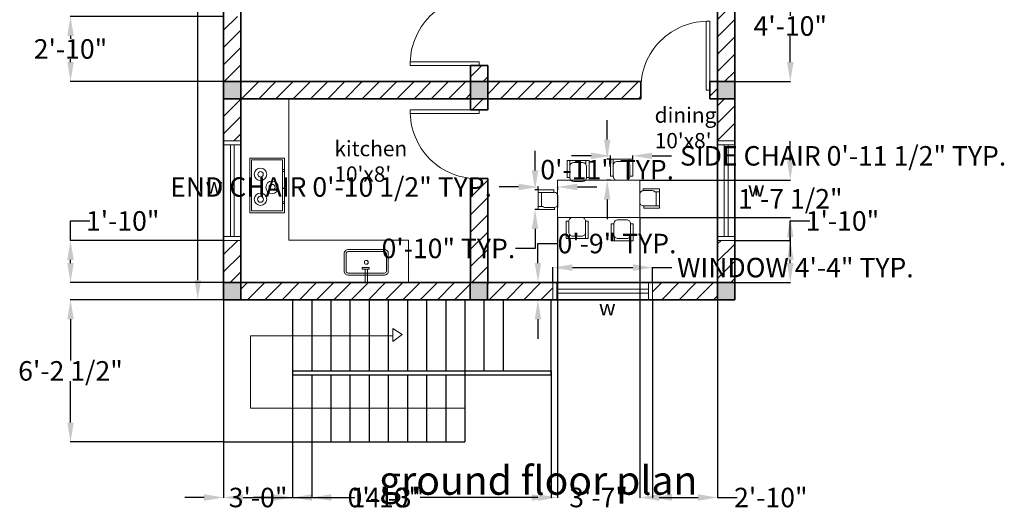
# Model space of a CAD drawing. Units: inches. Extents: x 1222 to 2611, y 176 to 793.
# Tile 1 of 5: x 1222 to 1737, y 176 to 433. Entities that reach past the tile are written whole.
import ezdxf

# ---------------------------------------------------------------- set-up
doc = ezdxf.new("R2010")
doc.units = ezdxf.units.IN
doc.header["$MEASUREMENT"] = 0
for name, color, linetype, lineweight in [('A-ANNO-DIMS', 2, 'Continuous', 18), ('A-ANNO-SYMB', 7, 'Continuous', 18), ('A-ANNO-TEXT', 7, 'Continuous', 25), ('A-AREA-IDEN', 7, 'Continuous', 25), ('A-COLS', 7, 'Continuous', 35), ('A-COLS-PATT', 18, 'Continuous', 13), ('A-DOOR', 3, 'Continuous', 18), ('A-EQPM', 8, 'Continuous', 18), ('A-FLOR-CASE', 9, 'Continuous', 18), ('A-FLOR-FIXT', 9, 'Continuous', 18), ('A-FLOR-STRS', 7, 'Continuous', 25), ('A-FURN', 8, 'Continuous', 18), ('A-GLAZ', 4, 'Continuous', 18), ('A-WALL', 7, 'Continuous', 35), ('A-WALL-PATT', 30, 'Continuous', 13)]:
    doc.layers.add(name, color=color, linetype=linetype, lineweight=lineweight)
doc.styles.get("Standard").update_dxf_attribs({"font": 'arial.ttf'})
doc.dimstyles.get("Standard").update_dxf_attribs({"dimtxt": 10.18, "dimasz": 10.18, "dimexe": 0.18, "dimexo": 0.0625, "dimgap": 0.09, "dimtad": 0, "dimtih": 1, "dimtoh": 1, "dimdec": 0, "dimzin": 0, "dimdsep": 46, "dimlunit": 3, "dimtxsty": 'Standard', "dimcen": 0.09, "dimadec": 0, "dimazin": 0, "dimtfac": 1, "dimtdec": 0, "dimtofl": 0, "dimtmove": 0, "dimatfit": 3, "dimfxl": 1, "dimtolj": 1, "dimtzin": 0, "dimarcsym": 0})

# ---------------------------------------------------------------- blocks, each defined once
blk = doc.blocks.new('*D10')
at = {"layer": 'A-ANNO-DIMS', "color": 0, "lineweight": -2, "transparency": 16777216}
for p, q in [((1328.74, 730.54), (1315.1, 730.54)), ((1315.28, 720.36), (1315.28, 513.8)), ((1315.28, 296.65), (1315.28, 503.21)), ((1328.74, 286.47), (1315.1, 286.47))]:
    blk.add_line(p, q, dxfattribs=at)
at = {"layer": 'A-ANNO-DIMS', "color": 0, "transparency": 16777216}
for points in [[(1313.58, 720.36), (1316.97, 720.36), (1315.28, 730.54)], [(1313.58, 296.65), (1316.97, 296.65), (1315.28, 286.47)]]:
    blk.add_solid(points, dxfattribs=at)
at = {"layer": 'Defpoints', "color": 0, "transparency": 16777216}
for p in [(1315.28, 730.54), (1328.8, 730.54), (1328.8, 286.47)]:
    blk.add_point(p, dxfattribs=at)
at = {"layer": 'A-ANNO-DIMS', "color": 0, "transparency": 16777216, "insert": (1315.28, 508.5), "char_height": 10.18, "attachment_point": 5}
blk.add_mtext("\\A1;37'", dxfattribs=at)
blk = doc.blocks.new('DOOR-SWING-36IN')
for p, q in [((34.01, 0), (34.01, 36)), ((36.01, 0), (36.01, 36)), ((34.01, 0), (36.01, 0))]:
    blk.add_line(p, q)
blk.add_arc((35.01, 1), 35.01, 88.3634, 181.6366)
blk = doc.blocks.new('WINDOW-48IN-PLAN')
for p, q in [((0, 0), (0, 9)), ((2, 0), (2, 9)), ((2, 5.5), (50, 5.5)), ((50, 0), (50, 9)), ((52, 0), (52, 9)), ((2, 3.5), (50, 3.5))]:
    blk.add_line(p, q)
blk = doc.blocks.new('COLUMN-9X9IN')
blk.add_lwpolyline([(0, 9), (9, 9), (9, 0), (0, 0)], close=True)
blk = doc.blocks.new('CHAIR-DINING-SIDE')
for points in [[(2.02, 10.94), (2.02, 10.94), (0, 10.94), (0, 10.94), (0, 4.9), (0, 4.9)], [(9.79, 9.21), (9.79, 9.21), (9.79, 10.94), (9.79, 10.94), (2.02, 10.94), (2.02, 10.94)], [(9.79, 8.89), (9.79, 10.94), (9.79, 10.94), (11.58, 10.94), (11.58, 10.94), (11.58, 2.01), (11.58, 2.01), (10.11, 2.01)]]:
    blk.add_lwpolyline(points)
blk.add_lwpolyline([(0, 10.94), (0, 10.94), (1.43, 10.94), (1.43, 10.94), (1.43, 2), (1.43, 2), (0, 2), (0, 2)], close=True)
blk.add_lwpolyline([(10.11, 2, -0.414214), (8.11, 0), (3.43, 0, -0.414214), (1.43, 2), (1.43, 7.79, -0.414214), (3.43, 9.79), (8.11, 9.79, -0.414214), (10.11, 7.79)], format="xyb", close=True)
blk = doc.blocks.new('CHAIR-DINING-END')
blk.add_lwpolyline([(2.18, 1.24), (2, 1.24, -0.414214), (0, 3.24), (0, 7.18, -0.414214), (2, 9.18), (6.51, 9.18, -0.198912), (7.92, 8.59)], format="xyb")
blk.add_lwpolyline([(1.78, 9.17), (1.78, 10.19), (1.78, 10.19), (10.36, 10.19), (10.36, 10.19), (10.36, 8.59), (10.36, 8.59), (7.92, 8.59)])
for points in [[(8.51, 8.59), (8.51, 8.59), (10.36, 8.59), (10.36, 8.59), (10.36, 1.33), (10.36, 1.33), (8.51, 1.33), (8.51, 1.33)], [(10.36, 1.33), (10.36, 1.33), (2.18, 1.33), (2.18, 1.33), (2.18, 0), (2.18, 0), (10.36, 0), (10.36, 0)]]:
    blk.add_lwpolyline(points, close=True)
blk = doc.blocks.new('*D18')
at = {"layer": 'A-ANNO-DIMS', "color": 0, "lineweight": -2, "transparency": 16777216}
for p, q in [((1500.8, 295.54), (1500.8, 303.45)), ((1510.98, 303.27), (1542.62, 303.27)), ((1552.8, 295.54), (1552.8, 303.45)), ((1552.8, 303.27), (1562.98, 303.27))]:
    blk.add_line(p, q, dxfattribs=at)
at = {"layer": 'A-ANNO-DIMS', "color": 0, "transparency": 16777216}
for points in [[(1510.98, 304.97), (1510.98, 301.58), (1500.8, 303.27)], [(1542.62, 304.97), (1542.62, 301.58), (1552.8, 303.27)]]:
    blk.add_solid(points, dxfattribs=at)
at = {"layer": 'Defpoints', "color": 0, "transparency": 16777216}
for p in [(1552.8, 303.27), (1500.8, 295.47), (1552.8, 295.47)]:
    blk.add_point(p, dxfattribs=at)
at = {"layer": 'A-ANNO-DIMS', "color": 0, "transparency": 16777216, "insert": (1627.48, 303.27), "char_height": 10.18, "attachment_point": 5}
blk.add_mtext('\\A1;WINDOW 4\'-4" TYP.', dxfattribs=at)
blk = doc.blocks.new('*D19')
at = {"layer": 'A-ANNO-DIMS', "color": 0, "lineweight": -2, "transparency": 16777216}
for p, q in [((1493, 305.65), (1493, 315.83)), ((1493, 315.83), (1503.18, 315.83)), ((1500.74, 295.47), (1492.82, 295.47)), ((1500.74, 286.47), (1492.82, 286.47)), ((1493, 276.29), (1493, 266.11))]:
    blk.add_line(p, q, dxfattribs=at)
at = {"layer": 'A-ANNO-DIMS', "color": 0, "transparency": 16777216}
for points in [[(1491.31, 305.65), (1494.7, 305.65), (1493, 295.47)], [(1491.31, 276.29), (1494.7, 276.29), (1493, 286.47)]]:
    blk.add_solid(points, dxfattribs=at)
at = {"layer": 'Defpoints', "color": 0, "transparency": 16777216}
for p in [(1493, 295.47), (1500.8, 295.47), (1500.8, 286.47)]:
    blk.add_point(p, dxfattribs=at)
at = {"layer": 'A-ANNO-DIMS', "color": 0, "transparency": 16777216, "insert": (1534.3, 315.83), "char_height": 10.18, "attachment_point": 5}
blk.add_mtext('\\A1;0\'-9" TYP.', dxfattribs=at)
blk = doc.blocks.new('*D22')
at = {"layer": 'A-ANNO-DIMS', "color": 0, "lineweight": -2, "transparency": 16777216}
for p, q in [((1520.73, 361.64), (1510.55, 361.64)), ((1530.91, 359.97), (1530.91, 361.82)), ((1542.48, 359.97), (1542.48, 361.82)), ((1552.66, 361.64), (1562.84, 361.64))]:
    blk.add_line(p, q, dxfattribs=at)
at = {"layer": 'A-ANNO-DIMS', "color": 0, "transparency": 16777216}
for points in [[(1520.73, 363.34), (1520.73, 359.95), (1530.91, 361.64)], [(1552.66, 363.34), (1552.66, 359.95), (1542.48, 361.64)]]:
    blk.add_solid(points, dxfattribs=at)
at = {"layer": 'Defpoints', "color": 0, "transparency": 16777216}
for p in [(1542.48, 361.64), (1530.91, 359.91), (1542.48, 359.91)]:
    blk.add_point(p, dxfattribs=at)
at = {"layer": 'A-ANNO-DIMS', "color": 0, "transparency": 16777216, "insert": (1652.42, 361.64), "char_height": 10.18, "attachment_point": 5}
blk.add_mtext('\\A1;SIDE CHAIR 0\'-11 1/2" TYP.', dxfattribs=at)
blk = doc.blocks.new('*D23')
at = {"layer": 'A-ANNO-DIMS', "color": 0, "lineweight": -2, "transparency": 16777216}
for p, q in [((1529.17, 370.09), (1529.17, 380.27)), ((1530.84, 359.91), (1528.99, 359.91)), ((1530.84, 348.96), (1528.99, 348.96)), ((1529.17, 338.78), (1529.17, 328.6))]:
    blk.add_line(p, q, dxfattribs=at)
at = {"layer": 'A-ANNO-DIMS', "color": 0, "transparency": 16777216}
for points in [[(1527.47, 370.09), (1530.87, 370.09), (1529.17, 359.91)], [(1527.47, 338.78), (1530.87, 338.78), (1529.17, 348.96)]]:
    blk.add_solid(points, dxfattribs=at)
at = {"layer": 'Defpoints', "color": 0, "transparency": 16777216}
for p in [(1529.17, 359.91), (1530.91, 359.91), (1530.91, 348.96)]:
    blk.add_point(p, dxfattribs=at)
at = {"layer": 'A-ANNO-DIMS', "color": 0, "transparency": 16777216, "insert": (1529.17, 354.43), "char_height": 10.18, "attachment_point": 5}
blk.add_mtext('\\A1;0\'-11" TYP.', dxfattribs=at)
blk = doc.blocks.new('*D24')
at = {"layer": 'A-ANNO-DIMS', "color": 0, "lineweight": -2, "transparency": 16777216}
for p, q in [((1482.85, 345.38), (1472.67, 345.38)), ((1493.03, 343.89), (1493.03, 345.56)), ((1503.39, 343.89), (1503.39, 345.56)), ((1513.57, 345.38), (1523.75, 345.38))]:
    blk.add_line(p, q, dxfattribs=at)
at = {"layer": 'A-ANNO-DIMS', "color": 0, "transparency": 16777216}
for points in [[(1482.85, 347.08), (1482.85, 343.68), (1493.03, 345.38)], [(1513.57, 347.08), (1513.57, 343.68), (1503.39, 345.38)]]:
    blk.add_solid(points, dxfattribs=at)
at = {"layer": 'Defpoints', "color": 0, "transparency": 16777216}
for p in [(1493.03, 345.38), (1493.03, 343.83), (1503.39, 343.83)]:
    blk.add_point(p, dxfattribs=at)
at = {"layer": 'A-ANNO-DIMS', "color": 0, "transparency": 16777216, "insert": (1384.92, 345.38), "char_height": 10.18, "attachment_point": 5}
blk.add_mtext('\\A1;END CHAIR 0\'-10 1/2" TYP.', dxfattribs=at)
blk = doc.blocks.new('*D25')
at = {"layer": 'A-ANNO-DIMS', "color": 0, "lineweight": -2, "transparency": 16777216}
for p, q in [((1491.48, 354.01), (1491.48, 364.19)), ((1492.97, 343.83), (1491.3, 343.83)), ((1492.97, 333.64), (1491.3, 333.64)), ((1491.48, 323.46), (1491.48, 313.28)), ((1491.48, 313.28), (1481.3, 313.28))]:
    blk.add_line(p, q, dxfattribs=at)
at = {"layer": 'A-ANNO-DIMS', "color": 0, "transparency": 16777216}
for points in [[(1489.78, 354.01), (1493.17, 354.01), (1491.48, 343.83)], [(1489.78, 323.46), (1493.17, 323.46), (1491.48, 333.64)]]:
    blk.add_solid(points, dxfattribs=at)
at = {"layer": 'Defpoints', "color": 0, "transparency": 16777216}
for p in [(1493.03, 343.83), (1491.48, 333.64), (1493.03, 333.64)]:
    blk.add_point(p, dxfattribs=at)
at = {"layer": 'A-ANNO-DIMS', "color": 0, "transparency": 16777216, "insert": (1446.22, 313.28), "char_height": 10.18, "attachment_point": 5}
blk.add_mtext('\\A1;0\'-10" TYP.', dxfattribs=at)
blk = doc.blocks.new('*D26')
at = {"layer": 'A-ANNO-DIMS', "color": 0, "lineweight": -2, "transparency": 16777216}
for p, q in [((1328.74, 286.47), (1248.62, 286.47)), ((1248.8, 276.29), (1248.8, 254.68)), ((1248.8, 222.35), (1248.8, 243.97)), ((1328.74, 212.17), (1248.62, 212.17))]:
    blk.add_line(p, q, dxfattribs=at)
at = {"layer": 'A-ANNO-DIMS', "color": 0, "transparency": 16777216}
for points in [[(1247.11, 276.29), (1250.5, 276.29), (1248.8, 286.47)], [(1247.11, 222.35), (1250.5, 222.35), (1248.8, 212.17)]]:
    blk.add_solid(points, dxfattribs=at)
at = {"layer": 'Defpoints', "color": 0, "transparency": 16777216}
for p in [(1328.8, 286.47), (1248.8, 212.17), (1328.8, 212.17)]:
    blk.add_point(p, dxfattribs=at)
at = {"layer": 'A-ANNO-DIMS', "color": 0, "transparency": 16777216, "insert": (1248.8, 249.32), "char_height": 10.18, "attachment_point": 5}
blk.add_mtext('\\A1;6\'-2 1/2"', dxfattribs=at)
blk = doc.blocks.new('*D27')
at = {"layer": 'A-ANNO-DIMS', "color": 0, "lineweight": -2, "transparency": 16777216}
for p, q in [((1328.8, 286.41), (1328.8, 182.99)), ((1499.95, 249.26), (1499.95, 182.99)), ((1338.98, 183.17), (1397.28, 183.17)), ((1489.77, 183.17), (1431.47, 183.17))]:
    blk.add_line(p, q, dxfattribs=at)
at = {"layer": 'A-ANNO-DIMS', "color": 0, "transparency": 16777216}
for points in [[(1338.98, 184.87), (1338.98, 181.47), (1328.8, 183.17)], [(1489.77, 184.87), (1489.77, 181.47), (1499.95, 183.17)]]:
    blk.add_solid(points, dxfattribs=at)
at = {"layer": 'Defpoints', "color": 0, "transparency": 16777216}
for p in [(1328.8, 286.47), (1499.95, 249.32), (1499.95, 183.17)]:
    blk.add_point(p, dxfattribs=at)
at = {"layer": 'A-ANNO-DIMS', "color": 0, "transparency": 16777216, "insert": (1414.38, 183.17), "char_height": 10.18, "attachment_point": 5}
blk.add_mtext('\\A1;14\'-3"', dxfattribs=at)
blk = doc.blocks.new('*D28')
at = {"layer": 'A-ANNO-DIMS', "color": 0, "lineweight": -2, "transparency": 16777216}
for p, q in [((1364.8, 212.11), (1364.8, 182.99)), ((1374.8, 212.11), (1374.8, 182.99)), ((1354.62, 183.17), (1344.44, 183.17)), ((1384.98, 183.17), (1395.16, 183.17))]:
    blk.add_line(p, q, dxfattribs=at)
at = {"layer": 'A-ANNO-DIMS', "color": 0, "transparency": 16777216}
for points in [[(1354.62, 184.87), (1354.62, 181.47), (1364.8, 183.17)], [(1384.98, 184.87), (1384.98, 181.47), (1374.8, 183.17)]]:
    blk.add_solid(points, dxfattribs=at)
at = {"layer": 'Defpoints', "color": 0, "transparency": 16777216}
for p in [(1364.8, 212.17), (1374.8, 212.17), (1374.8, 183.17)]:
    blk.add_point(p, dxfattribs=at)
at = {"layer": 'A-ANNO-DIMS', "color": 0, "transparency": 16777216, "insert": (1412.74, 183.17), "char_height": 10.18, "attachment_point": 5}
blk.add_mtext('\\A1;0\'-10"', dxfattribs=at)
blk = doc.blocks.new('*D29')
at = {"layer": 'A-ANNO-DIMS', "color": 0, "lineweight": -2, "transparency": 16777216}
for p, q in [((1328.8, 212.11), (1328.8, 182.99)), ((1364.8, 212.11), (1364.8, 182.99)), ((1318.62, 183.17), (1308.44, 183.17)), ((1374.98, 183.17), (1385.16, 183.17))]:
    blk.add_line(p, q, dxfattribs=at)
at = {"layer": 'A-ANNO-DIMS', "color": 0, "transparency": 16777216}
for points in [[(1318.62, 184.87), (1318.62, 181.47), (1328.8, 183.17)], [(1374.98, 184.87), (1374.98, 181.47), (1364.8, 183.17)]]:
    blk.add_solid(points, dxfattribs=at)
at = {"layer": 'Defpoints', "color": 0, "transparency": 16777216}
for p in [(1328.8, 212.17), (1364.8, 212.17), (1328.8, 183.17)]:
    blk.add_point(p, dxfattribs=at)
at = {"layer": 'A-ANNO-DIMS', "color": 0, "transparency": 16777216, "insert": (1346.8, 183.17), "char_height": 10.18, "attachment_point": 5}
blk.add_mtext('\\A1;3\'-0"', dxfattribs=at)
blk = doc.blocks.new('*D34')
at = {"layer": 'A-ANNO-DIMS', "color": 0, "lineweight": -2, "transparency": 16777216}
for p, q in [((1328.74, 434.47), (1248.62, 434.47)), ((1248.8, 424.29), (1248.8, 422.76)), ((1248.8, 410.65), (1248.8, 412.19)), ((1328.74, 400.47), (1248.62, 400.47))]:
    blk.add_line(p, q, dxfattribs=at)
at = {"layer": 'A-ANNO-DIMS', "color": 0, "transparency": 16777216}
for points in [[(1247.11, 424.29), (1250.5, 424.29), (1248.8, 434.47)], [(1247.11, 410.65), (1250.5, 410.65), (1248.8, 400.47)]]:
    blk.add_solid(points, dxfattribs=at)
at = {"layer": 'Defpoints', "color": 0, "transparency": 16777216}
for p in [(1248.8, 434.47), (1328.8, 434.47), (1328.8, 400.47)]:
    blk.add_point(p, dxfattribs=at)
at = {"layer": 'A-ANNO-DIMS', "color": 0, "transparency": 16777216, "insert": (1248.8, 417.47), "char_height": 10.18, "attachment_point": 5}
blk.add_mtext('\\A1;2\'-10"', dxfattribs=at)
blk = doc.blocks.new('*D35')
at = {"layer": 'A-ANNO-DIMS', "color": 0, "lineweight": -2, "transparency": 16777216}
for p, q in [((1248.8, 317.47), (1248.8, 327.65)), ((1248.8, 327.65), (1258.98, 327.65)), ((1328.74, 317.47), (1248.62, 317.47)), ((1248.8, 305.65), (1248.8, 307.29)), ((1337.74, 295.47), (1248.62, 295.47))]:
    blk.add_line(p, q, dxfattribs=at)
at = {"layer": 'A-ANNO-DIMS', "color": 0, "transparency": 16777216}
for points in [[(1247.11, 307.29), (1250.5, 307.29), (1248.8, 317.47)], [(1247.11, 305.65), (1250.5, 305.65), (1248.8, 295.47)]]:
    blk.add_solid(points, dxfattribs=at)
at = {"layer": 'Defpoints', "color": 0, "transparency": 16777216}
for p in [(1248.8, 317.47), (1328.8, 317.47), (1337.8, 295.47)]:
    blk.add_point(p, dxfattribs=at)
at = {"layer": 'A-ANNO-DIMS', "color": 0, "transparency": 16777216, "insert": (1276.08, 327.65), "char_height": 10.18, "attachment_point": 5}
blk.add_mtext('\\A1;1\'-10"', dxfattribs=at)
blk = doc.blocks.new('*D36')
at = {"layer": 'A-ANNO-DIMS', "color": 0, "lineweight": -2, "transparency": 16777216}
for p, q in [((1595.87, 458.47), (1624.98, 458.47)), ((1624.8, 448.29), (1624.8, 434.73)), ((1624.8, 410.59), (1624.8, 424.15)), ((1595.87, 400.41), (1624.98, 400.41))]:
    blk.add_line(p, q, dxfattribs=at)
at = {"layer": 'A-ANNO-DIMS', "color": 0, "transparency": 16777216}
for points in [[(1623.11, 448.29), (1626.5, 448.29), (1624.8, 458.47)], [(1623.11, 410.59), (1626.5, 410.59), (1624.8, 400.41)]]:
    blk.add_solid(points, dxfattribs=at)
at = {"layer": 'Defpoints', "color": 0, "transparency": 16777216}
for p in [(1595.8, 458.47), (1624.8, 458.47), (1595.8, 400.41)]:
    blk.add_point(p, dxfattribs=at)
at = {"layer": 'A-ANNO-DIMS', "color": 0, "transparency": 16777216, "insert": (1624.8, 429.44), "char_height": 10.18, "attachment_point": 5}
blk.add_mtext('\\A1;4\'-10"', dxfattribs=at)
blk = doc.blocks.new('*D38')
at = {"layer": 'A-ANNO-DIMS', "color": 0, "lineweight": -2, "transparency": 16777216}
for p, q in [((1624.8, 317.47), (1624.8, 327.65)), ((1624.8, 327.65), (1634.98, 327.65)), ((1595.87, 317.47), (1624.98, 317.47)), ((1624.8, 305.65), (1624.8, 307.29)), ((1586.87, 295.47), (1624.98, 295.47))]:
    blk.add_line(p, q, dxfattribs=at)
at = {"layer": 'A-ANNO-DIMS', "color": 0, "transparency": 16777216}
for points in [[(1623.11, 307.29), (1626.5, 307.29), (1624.8, 317.47)], [(1623.11, 305.65), (1626.5, 305.65), (1624.8, 295.47)]]:
    blk.add_solid(points, dxfattribs=at)
at = {"layer": 'Defpoints', "color": 0, "transparency": 16777216}
for p in [(1595.8, 317.47), (1624.8, 317.47), (1586.8, 295.47)]:
    blk.add_point(p, dxfattribs=at)
at = {"layer": 'A-ANNO-DIMS', "color": 0, "transparency": 16777216, "insert": (1652.08, 327.65), "char_height": 10.18, "attachment_point": 5}
blk.add_mtext('\\A1;1\'-10"', dxfattribs=at)
blk = doc.blocks.new('*D39')
at = {"layer": 'A-ANNO-DIMS', "color": 0, "lineweight": -2, "transparency": 16777216}
for p, q in [((1586.8, 295.41), (1586.8, 182.99)), ((1552.8, 286.41), (1552.8, 182.99)), ((1562.98, 183.17), (1576.62, 183.17)), ((1586.8, 183.17), (1596.98, 183.17))]:
    blk.add_line(p, q, dxfattribs=at)
at = {"layer": 'A-ANNO-DIMS', "color": 0, "transparency": 16777216}
for points in [[(1562.98, 184.87), (1562.98, 181.47), (1552.8, 183.17)], [(1576.62, 184.87), (1576.62, 181.47), (1586.8, 183.17)]]:
    blk.add_solid(points, dxfattribs=at)
at = {"layer": 'Defpoints', "color": 0, "transparency": 16777216}
for p in [(1586.8, 295.47), (1552.8, 286.47), (1586.8, 183.17)]:
    blk.add_point(p, dxfattribs=at)
at = {"layer": 'A-ANNO-DIMS', "color": 0, "transparency": 16777216, "insert": (1614.65, 183.17), "char_height": 10.18, "attachment_point": 5}
blk.add_mtext('\\A1;2\'-10"', dxfattribs=at)
blk = doc.blocks.new('*D40')
at = {"layer": 'A-ANNO-DIMS', "color": 0, "lineweight": -2, "transparency": 16777216}
for p, q in [((1503.19, 329.39), (1503.19, 182.99)), ((1546.16, 329.39), (1546.16, 182.99)), ((1493.01, 183.17), (1482.83, 183.17)), ((1556.34, 183.17), (1566.52, 183.17))]:
    blk.add_line(p, q, dxfattribs=at)
at = {"layer": 'A-ANNO-DIMS', "color": 0, "transparency": 16777216}
for points in [[(1493.01, 184.87), (1493.01, 181.47), (1503.19, 183.17)], [(1556.34, 184.87), (1556.34, 181.47), (1546.16, 183.17)]]:
    blk.add_solid(points, dxfattribs=at)
at = {"layer": 'Defpoints', "color": 0, "transparency": 16777216}
for p in [(1503.19, 329.45), (1546.16, 329.45), (1546.16, 183.17)]:
    blk.add_point(p, dxfattribs=at)
at = {"layer": 'A-ANNO-DIMS', "color": 0, "transparency": 16777216, "insert": (1524.67, 183.17), "char_height": 10.18, "attachment_point": 5}
blk.add_mtext('\\A1;3\'-7"', dxfattribs=at)
blk = doc.blocks.new('*D41')
at = {"layer": 'A-ANNO-DIMS', "color": 0, "lineweight": -2, "transparency": 16777216}
for p, q in [((1624.8, 359.14), (1624.8, 369.32)), ((1546.22, 348.96), (1624.98, 348.96)), ((1546.22, 329.45), (1624.98, 329.45)), ((1624.8, 319.27), (1624.8, 309.09))]:
    blk.add_line(p, q, dxfattribs=at)
at = {"layer": 'A-ANNO-DIMS', "color": 0, "transparency": 16777216}
for points in [[(1623.11, 359.14), (1626.5, 359.14), (1624.8, 348.96)], [(1623.11, 319.27), (1626.5, 319.27), (1624.8, 329.45)]]:
    blk.add_solid(points, dxfattribs=at)
at = {"layer": 'Defpoints', "color": 0, "transparency": 16777216}
for p in [(1546.16, 348.96), (1624.8, 348.96), (1546.16, 329.45)]:
    blk.add_point(p, dxfattribs=at)
at = {"layer": 'A-ANNO-DIMS', "color": 0, "transparency": 16777216, "insert": (1624.8, 339.21), "char_height": 10.18, "attachment_point": 5}
blk.add_mtext('\\A1;1\'-7 1/2"', dxfattribs=at)

msp = doc.modelspace()

# ---------------------------------------------------------------- hatches: boundary and pattern name
at = {"layer": 'A-COLS-PATT'}
h = msp.add_hatch(color=256, dxfattribs=at)
h.dxf.hatch_style = 1
h.paths.add_polyline_path([(1337.8, 730.47), (1328.8, 730.47), (1328.8, 721.47), (1337.8, 721.47)])
h.paths.add_polyline_path([(1466.8, 730.47), (1457.8, 730.47), (1457.8, 721.47), (1466.8, 721.47)])
h.paths.add_polyline_path([(1595.8, 730.47), (1586.8, 730.47), (1586.8, 721.47), (1595.8, 721.47)])
h.paths.add_polyline_path([(1595.8, 601.42), (1586.8, 601.42), (1586.8, 592.42), (1595.8, 592.42)])
h.paths.add_polyline_path([(1466.8, 601.47), (1457.8, 601.47), (1457.8, 592.47), (1466.8, 592.47)])
h.paths.add_polyline_path([(1337.8, 601.47), (1328.8, 601.47), (1328.8, 592.47), (1337.8, 592.47)])
h.paths.add_polyline_path([(1337.8, 400.47), (1328.8, 400.47), (1328.8, 391.47), (1337.8, 391.47)])
h.paths.add_polyline_path([(1466.8, 400.47), (1457.8, 400.47), (1457.8, 391.47), (1466.8, 391.47)])
h.paths.add_polyline_path([(1595.8, 400.41), (1586.8, 400.41), (1586.8, 391.41), (1595.8, 391.41)])
h.paths.add_polyline_path([(1466.56, 295.47), (1457.56, 295.47), (1457.56, 286.47), (1466.56, 286.47)])
h.paths.add_polyline_path([(1595.8, 295.47), (1586.8, 295.47), (1586.8, 286.47), (1595.8, 286.47)])
h.paths.add_polyline_path([(1337.8, 295.47), (1328.8, 295.47), (1328.8, 286.47), (1337.8, 286.47)])
at = {"layer": 'A-WALL-PATT'}
h = msp.add_hatch(dxfattribs=at)
h.set_pattern_fill('ANSI31', color=256, scale=51)
h.paths.add_polyline_path([(1337.8, 721.47), (1328.8, 721.47), (1328.8, 687.47), (1337.8, 687.47)])
h.paths.add_polyline_path([(1337.8, 635.47), (1328.8, 635.47), (1328.8, 601.47), (1337.8, 601.47)])
h.paths.add_polyline_path([(1371.8, 730.47), (1337.8, 730.47), (1337.8, 721.47), (1371.8, 721.47)])
h.paths.add_polyline_path([(1457.8, 730.47), (1423.8, 730.47), (1423.8, 721.47), (1457.8, 721.47)])
h.paths.add_polyline_path([(1466.8, 721.47), (1457.8, 721.47), (1457.8, 601.47), (1466.8, 601.47)])
h.paths.add_polyline_path([(1539.2, 596.97, -0.014283), (1539.2, 598.97), (1539.2, 601.47), (1466.8, 601.47), (1466.8, 592.47), (1539.2, 592.47)])
h.paths.add_polyline_path([(1595.8, 592.42), (1586.8, 592.42), (1586.8, 534.47), (1595.8, 534.47)])
h.paths.add_polyline_path([(1595.8, 458.47), (1586.8, 458.47), (1586.8, 400.41), (1595.8, 400.41)])
h.paths.add_polyline_path([(1595.8, 391.41), (1586.8, 391.41), (1586.8, 369.47), (1595.8, 369.47)])
h.paths.add_polyline_path([(1595.8, 317.47), (1586.8, 317.47), (1586.8, 295.47), (1595.8, 295.47)])
h.paths.add_polyline_path([(1586.8, 295.47), (1552.8, 295.47), (1552.8, 286.47), (1586.8, 286.47)])
h.paths.add_polyline_path([(1500.8, 295.47), (1466.8, 295.47), (1466.8, 349.72), (1462.3, 349.72, -0.014283), (1460.3, 349.72), (1457.8, 349.72), (1457.8, 295.47), (1466.56, 295.47), (1466.56, 286.47), (1500.8, 286.47)])
h.paths.add_polyline_path([(1457.56, 295.47), (1337.8, 295.47), (1337.8, 286.47), (1457.56, 286.47)])
h.paths.add_polyline_path([(1337.8, 317.47), (1328.8, 317.47), (1328.8, 295.47), (1337.8, 295.47)])
h.paths.add_polyline_path([(1337.8, 391.47), (1328.8, 391.47), (1328.8, 369.47), (1337.8, 369.47)])
h.paths.add_polyline_path([(1337.8, 434.47), (1328.8, 434.47), (1328.8, 400.47), (1337.8, 400.47)])
h.paths.add_polyline_path([(1457.8, 400.47), (1337.8, 400.47), (1337.8, 391.47), (1457.8, 391.47)])
h.paths.add_polyline_path([(1546.8, 395.97, -0.014283), (1546.8, 397.97), (1546.8, 400.47), (1466.8, 400.47), (1466.8, 391.47), (1546.8, 391.47)])
h.paths.add_polyline_path([(1466.8, 408.77), (1457.8, 408.77), (1457.8, 400.47), (1466.8, 400.47)])
h.paths.add_polyline_path([(1466.8, 391.47), (1457.8, 391.47), (1457.8, 385.72), (1466.8, 385.72)])
h.paths.add_polyline_path([(1586.8, 400.47), (1582.8, 400.47), (1582.8, 395.97), (1582.8, 391.47), (1586.8, 391.47)])
h.paths.add_polyline_path([(1466.8, 529.47), (1457.8, 529.47), (1406.8, 529.47), (1406.8, 592.47), (1414.87, 592.47), (1414.87, 596.97, -0.014283), (1414.87, 598.97), (1414.87, 601.47), (1375.45, 601.47), (1375.45, 598.97, -0.017236), (1375.45, 596.97), (1375.45, 592.47), (1397.8, 592.47), (1397.8, 529.47), (1337.8, 529.47), (1337.8, 546.97), (1328.8, 546.97), (1328.8, 486.47), (1337.8, 486.47), (1337.8, 490.02), (1337.8, 520.47), (1457.8, 520.47), (1457.8, 444.77), (1460.3, 444.77, -0.014283), (1462.3, 444.77), (1466.8, 444.77)])
h.paths.add_polyline_path([(1457.8, 601.47), (1450.87, 601.47), (1450.87, 596.97), (1450.87, 592.47), (1457.8, 592.47)], flags=0)
h.paths.add_polyline_path([(1586.8, 601.47), (1575.2, 601.47), (1575.2, 596.97), (1575.2, 592.47), (1586.8, 592.47)])

# ---------------------------------------------------------------- linework, layer by layer
at = {"layer": 'A-ANNO-SYMB'}
for p, q in [((1342.91, 229.91), (1342.91, 267.63)), ((1342.91, 267.63), (1417.15, 267.63)), ((1417.15, 267.63), (1417.15, 271.4)), ((1417.15, 271.4), (1417.15, 264.58)), ((1422.14, 268.32), (1417.15, 271.4)), ((1417.15, 264.58), (1422.14, 268.32)), ((1454.8, 229.91), (1342.91, 229.91))]:
    msp.add_line(p, q, dxfattribs=at)
at = {"layer": 'A-EQPM'}
for points in [[(1342.4, 360.49), (1360.56, 360.49), (1360.56, 331.92), (1342.4, 331.92)], [(1343.4, 359.49), (1359.56, 359.49), (1359.56, 332.92), (1343.4, 332.92)], [(1359.56, 354.42), (1360.56, 354.42), (1360.56, 353.46), (1359.56, 353.46)], [(1359.56, 344.54), (1360.56, 344.54), (1360.56, 344.83), (1359.56, 344.83)], [(1359.56, 337.62), (1360.56, 337.62), (1360.56, 336.82), (1359.56, 336.82)]]:
    msp.add_lwpolyline(points, close=True, dxfattribs=at)
for centre, radius in [((1348.06, 351.98), 3.23), ((1348.06, 351.98), 1.42), ((1354.08, 345.19), 3.23), ((1354.08, 345.19), 1.56), ((1348.06, 338.95), 3.23), ((1348.06, 338.95), 1.59)]:
    msp.add_circle(centre, radius, dxfattribs=at)
at = {"layer": 'A-FLOR-CASE'}
for p, q in [((1362.88, 391.47), (1362.88, 317.56)), ((1362.88, 317.56), (1425.32, 317.56)), ((1425.32, 317.56), (1425.32, 295.47))]:
    msp.add_line(p, q, dxfattribs=at)
at = {"layer": 'A-FLOR-FIXT'}
for points in [[(1391.79, 310.65, -0.414214), (1393.79, 312.65), (1412.83, 312.65, -0.414214), (1414.83, 310.65), (1414.83, 301.37, -0.414214), (1412.83, 299.37), (1393.79, 299.37, -0.414214), (1391.79, 301.37)], [(1392.79, 310.65, -0.414214), (1393.79, 311.65), (1412.83, 311.65, -0.414214), (1413.83, 310.65), (1413.83, 301.37, -0.414214), (1412.83, 300.37), (1393.79, 300.37, -0.414214), (1392.79, 301.37)]]:
    msp.add_lwpolyline(points, format="xyb", close=True, dxfattribs=at)
for points in [[(1401.25, 302.44), (1401.25, 302.44), (1404.9, 302.44), (1404.9, 302.44), (1404.9, 303.35), (1404.9, 303.35), (1401.25, 303.35), (1401.25, 303.35)], [(1402.76, 302.44), (1402.76, 302.44), (1404.01, 302.44), (1404.01, 302.44), (1404.01, 295.47), (1404.01, 295.47), (1402.76, 295.47), (1402.76, 295.47)]]:
    msp.add_lwpolyline(points, close=True, dxfattribs=at)
msp.add_circle((1403.31, 306.01), 0.996, dxfattribs=at)
at = {"layer": 'A-FLOR-STRS'}
for p, q in [((1328.8, 286.47), (1328.8, 212.17)), ((1364.8, 286.47), (1364.8, 212.17)), ((1374.8, 286.47), (1374.8, 249.32)), ((1384.8, 286.47), (1384.8, 249.32)), ((1394.8, 286.47), (1394.8, 249.32)), ((1404.8, 286.47), (1404.8, 249.32)), ((1414.8, 286.47), (1414.8, 249.32)), ((1424.8, 286.47), (1424.8, 249.32)), ((1434.8, 286.47), (1434.8, 249.32)), ((1444.8, 286.47), (1444.8, 249.32)), ((1454.8, 286.47), (1454.8, 212.17)), ((1464.8, 286.47), (1464.8, 249.32)), ((1474.8, 286.47), (1474.8, 249.32)), ((1499.95, 247.32), (1499.95, 286.47)), ((1364.8, 249.32), (1499.95, 249.32)), ((1364.8, 247.32), (1499.95, 247.32)), ((1374.8, 247.32), (1374.8, 212.17)), ((1384.8, 247.32), (1384.8, 212.17)), ((1394.8, 247.32), (1394.8, 212.17)), ((1404.8, 247.32), (1404.8, 212.17)), ((1414.8, 247.32), (1414.8, 212.17)), ((1424.8, 247.32), (1424.8, 212.17)), ((1434.8, 247.32), (1434.8, 212.17)), ((1444.8, 247.32), (1444.8, 212.17)), ((1328.8, 212.17), (1454.8, 212.17))]:
    msp.add_line(p, q, dxfattribs=at)
at = {"layer": 'A-FURN'}
for points in [[(1532.92, 358.17), (1532.92, 358.17)], [(1503.19, 348.96), (1503.19, 348.96), (1546.16, 348.96), (1546.16, 348.96), (1546.16, 329.45), (1546.16, 329.45), (1503.19, 329.45), (1503.19, 329.45)], [(1503.19, 348.96), (1503.19, 348.96), (1546.16, 348.96), (1546.16, 348.96), (1546.16, 329.45), (1546.16, 329.45), (1503.19, 329.45), (1503.19, 329.45)], [(1547.94, 342.87), (1547.94, 342.87)]]:
    msp.add_lwpolyline(points, close=True, dxfattribs=at)
for points in [[(1554.67, 341.45), (1554.67, 337.51)], [(1503.39, 338.62), (1503.39, 334.68)]]:
    msp.add_lwpolyline(points, dxfattribs=at)
at = {"layer": 'A-GLAZ'}
msp.add_line((1334.3, 367.47), (1334.3, 319.47), dxfattribs=at)
at = {"layer": 'A-WALL'}
for p, q in [((1328.8, 286.47), (1328.8, 730.47)), ((1595.8, 730.47), (1595.8, 286.47)), ((1586.8, 592.47), (1586.8, 400.47)), ((1337.8, 400.47), (1337.8, 520.47)), ((1457.8, 400.47), (1457.8, 408.77)), ((1457.8, 408.77), (1466.8, 408.77)), ((1466.8, 400.47), (1466.8, 408.77)), ((1337.8, 400.47), (1457.8, 400.47)), ((1466.8, 400.47), (1546.8, 400.47)), ((1546.8, 395.97), (1546.8, 400.47)), ((1582.8, 400.47), (1582.8, 391.47)), ((1582.8, 400.47), (1586.8, 400.47)), ((1337.8, 295.47), (1337.8, 391.47)), ((1337.8, 391.47), (1457.8, 391.47)), ((1457.8, 385.72), (1457.8, 391.47)), ((1466.8, 391.47), (1546.8, 391.47)), ((1466.8, 385.72), (1466.8, 391.47)), ((1546.8, 395.97), (1546.8, 391.47)), ((1582.8, 391.47), (1586.8, 391.47)), ((1586.8, 391.47), (1586.8, 295.47)), ((1457.8, 385.72), (1466.8, 385.72)), ((1457.8, 295.47), (1457.8, 349.72)), ((1462.3, 349.72), (1457.8, 349.72)), ((1462.3, 349.72), (1466.8, 349.72)), ((1466.8, 295.47), (1466.8, 349.72)), ((1457.8, 295.47), (1337.8, 295.47)), ((1586.8, 295.47), (1466.8, 295.47)), ((1595.8, 286.47), (1328.8, 286.47))]:
    msp.add_line(p, q, dxfattribs=at)

# ---------------------------------------------------------------- block references
at = {"layer": 'A-COLS'}
for p in [(1328.8, 391.47), (1457.8, 391.47), (1586.8, 391.41), (1328.8, 286.47), (1457.56, 286.47), (1586.8, 286.47)]:
    msp.add_blockref('COLUMN-9X9IN', p, dxfattribs=at)
at = {"layer": 'A-DOOR', "extrusion": (0, 0, -1), "zscale": -1, "rotation": 270.0000000000005}
msp.add_blockref('DOOR-SWING-36IN', (-1462.3, 444.78), dxfattribs=at)
at = {"layer": 'A-DOOR'}
msp.add_blockref('DOOR-SWING-36IN', (1546.78, 395.97), dxfattribs=at)
at = {"layer": 'A-DOOR', "rotation": 90.00000000000055}
msp.add_blockref('DOOR-SWING-36IN', (1462.3, 349.71), dxfattribs=at)
at = {"layer": 'A-FURN'}
for name, p in [('CHAIR-DINING-SIDE', (1508.23, 348.3)), ('CHAIR-DINING-SIDE', (1530.91, 348.96)), ('CHAIR-DINING-END', (1546.16, 334.28))]:
    msp.add_blockref(name, p, dxfattribs=at)
at = {"layer": 'A-FURN', "rotation": 180}
for name, p in [('CHAIR-DINING-END', (1503.39, 343.83)), ('CHAIR-DINING-SIDE', (1519.28, 329.45)), ('CHAIR-DINING-SIDE', (1542.82, 328.2))]:
    msp.add_blockref(name, p, dxfattribs=at)
at = {"layer": 'A-GLAZ'}
for p, rotation in [((1337.8, 317.47), 89.99999999999888), ((1595.8, 317.47), 89.99999999999937)]:
    msp.add_blockref('WINDOW-48IN-PLAN', p, dxfattribs=dict(at, rotation=rotation))
msp.add_blockref('WINDOW-48IN-PLAN', (1500.8, 286.47), dxfattribs=at)

# ---------------------------------------------------------------- texts
at = {"layer": 'A-ANNO-TEXT', "attachment_point": 1}
for s, width, insert, char_height in [('w', 4.8776, (1319.47, 349.97), 8), ('w', 4.8776, (1602.65, 348.36), 8), ('w', 4.8776, (1524.83, 286.36), 8), ('ground floor plan', 302.9253, (1409.95, 199.6), 15)]:
    msp.add_mtext_dynamic_manual_height_columns(s, width=width, gutter_width=1, heights=[0], dxfattribs=dict(at, insert=insert, char_height=char_height))
at = {"layer": 'A-AREA-IDEN', "char_height": 8, "attachment_point": 1}
for s, insert in [("dining\\P10'x8'", (1553.97, 386.91)), ("kitchen\\P10'x8'", (1386.65, 369.45))]:
    msp.add_mtext_dynamic_manual_height_columns(s, width=78.0148, gutter_width=1, heights=[0], dxfattribs=dict(at, insert=insert))

# ---------------------------------------------------------------- dimensions: what is measured, and where the dimension line sits
at = {"layer": 'A-ANNO-DIMS'}
for base, p1, p2, override, picture, middle in [((1315.28, 730.54), (1328.8, 286.47), (1328.8, 730.54), {"dimclrd": 0, "dimclre": 0, "dimclrt": 0}, '*D10', (1315.28, 508.5)), ((1624.8, 458.47), (1595.8, 400.41), (1595.8, 458.47), {"dimdec": 1, "dimlfac": 1, "dimrnd": 0, "dimzin": 1, "dimdsep": 46, "dimlunit": 4, "dimfrac": 2}, '*D36', (1624.8, 429.44)), ((1248.8, 434.47), (1328.8, 400.47), (1328.8, 434.47), {"dimdec": 1, "dimlfac": 1, "dimrnd": 0, "dimzin": 1, "dimdsep": 46, "dimlunit": 4, "dimfrac": 2}, '*D34', (1248.8, 417.47)), ((1624.8, 348.96), (1546.16, 329.45), (1546.16, 348.96), {"dimdec": 1, "dimlfac": 1, "dimrnd": 0, "dimzin": 1, "dimdsep": 46, "dimlunit": 4, "dimfrac": 2}, '*D41', (1624.8, 339.21)), ((1248.8, 317.47), (1337.8, 295.47), (1328.8, 317.47), {"dimdec": 1, "dimlfac": 1, "dimrnd": 0, "dimzin": 1, "dimdsep": 46, "dimlunit": 4, "dimfrac": 2}, '*D35', (1276.08, 327.65)), ((1624.8, 317.47), (1586.8, 295.47), (1595.8, 317.47), {"dimdec": 1, "dimlfac": 1, "dimrnd": 0, "dimzin": 1, "dimdsep": 46, "dimlunit": 4, "dimfrac": 2}, '*D38', (1652.08, 327.65)), ((1248.8, 212.17), (1328.8, 286.47), (1328.8, 212.17), {"dimdec": 1, "dimlfac": 1, "dimrnd": 0, "dimzin": 1, "dimdsep": 46, "dimlunit": 4, "dimfrac": 2}, '*D26', (1248.8, 249.32))]:
    dim = msp.add_linear_dim(base=base, p1=p1, p2=p2, angle=90, dimstyle='Standard', override=override, dxfattribs=at)
    dim.commit()
    dim.dimension.update_dxf_attribs({"geometry": picture, "text_midpoint": middle})
for base, p1, p2, text, picture, middle in [((1542.48, 361.64), (1530.91, 359.91), (1542.48, 359.91), 'SIDE CHAIR <> TYP.', '*D22', (1652.42, 361.64)), ((1552.8, 303.27), (1500.8, 295.47), (1552.8, 295.47), 'WINDOW <> TYP.', '*D18', (1627.48, 303.27))]:
    dim = msp.add_linear_dim(base=base, p1=p1, p2=p2, text=text, dimstyle='Standard', override={"dimdec": 1, "dimlfac": 1, "dimrnd": 0, "dimzin": 1, "dimdsep": 46, "dimlunit": 4, "dimfrac": 2}, dxfattribs=at)
    dim.commit()
    dim.dimension.update_dxf_attribs({"geometry": picture, "text_midpoint": middle})
for base, p1, p2, angle, text, picture, middle in [((1493.03, 345.38), (1503.39, 343.83), (1493.03, 343.83), 180, 'END CHAIR <> TYP.', '*D24', (1384.92, 345.38)), ((1529.1685, 359.9064), (1530.9052, 348.9627), (1530.9052, 359.9064), 90, '<> TYP.', '*D23', (1529.1685, 354.4346)), ((1491.48, 333.64), (1493.03, 343.83), (1493.03, 333.64), 270, '<> TYP.', '*D25', (1446.22, 313.28)), ((1493, 295.47), (1500.8, 286.47), (1500.8, 295.47), 90, '<> TYP.', '*D19', (1534.3, 315.83))]:
    dim = msp.add_linear_dim(base=base, p1=p1, p2=p2, angle=angle, text=text, dimstyle='Standard', override={"dimdec": 1, "dimlfac": 1, "dimrnd": 0, "dimzin": 1, "dimdsep": 46, "dimlunit": 4, "dimfrac": 2}, dxfattribs=at)
    dim.commit()
    dim.dimension.update_dxf_attribs({"geometry": picture, "text_midpoint": middle})
for base, p1, p2, picture, middle in [((1546.16, 183.17), (1503.19, 329.45), (1546.16, 329.45), '*D40', (1524.67, 183.17)), ((1586.8, 183.17), (1552.8, 286.47), (1586.8, 295.47), '*D39', (1614.65, 183.17)), ((1499.9512, 183.1706), (1328.8046, 286.4733), (1499.9512, 249.322), '*D27', (1414.3779, 183.1706)), ((1328.8, 183.17), (1364.8, 212.17), (1328.8, 212.17), '*D29', (1346.8, 183.17)), ((1374.8, 183.17), (1364.8, 212.17), (1374.8, 212.17), '*D28', (1412.74, 183.17))]:
    dim = msp.add_linear_dim(base=base, p1=p1, p2=p2, dimstyle='Standard', override={"dimdec": 1, "dimlfac": 1, "dimrnd": 0, "dimzin": 1, "dimdsep": 46, "dimlunit": 4, "dimfrac": 2}, dxfattribs=at)
    dim.commit()
    dim.dimension.update_dxf_attribs({"geometry": picture, "text_midpoint": middle})

doc.saveas('drawing.dxf')
